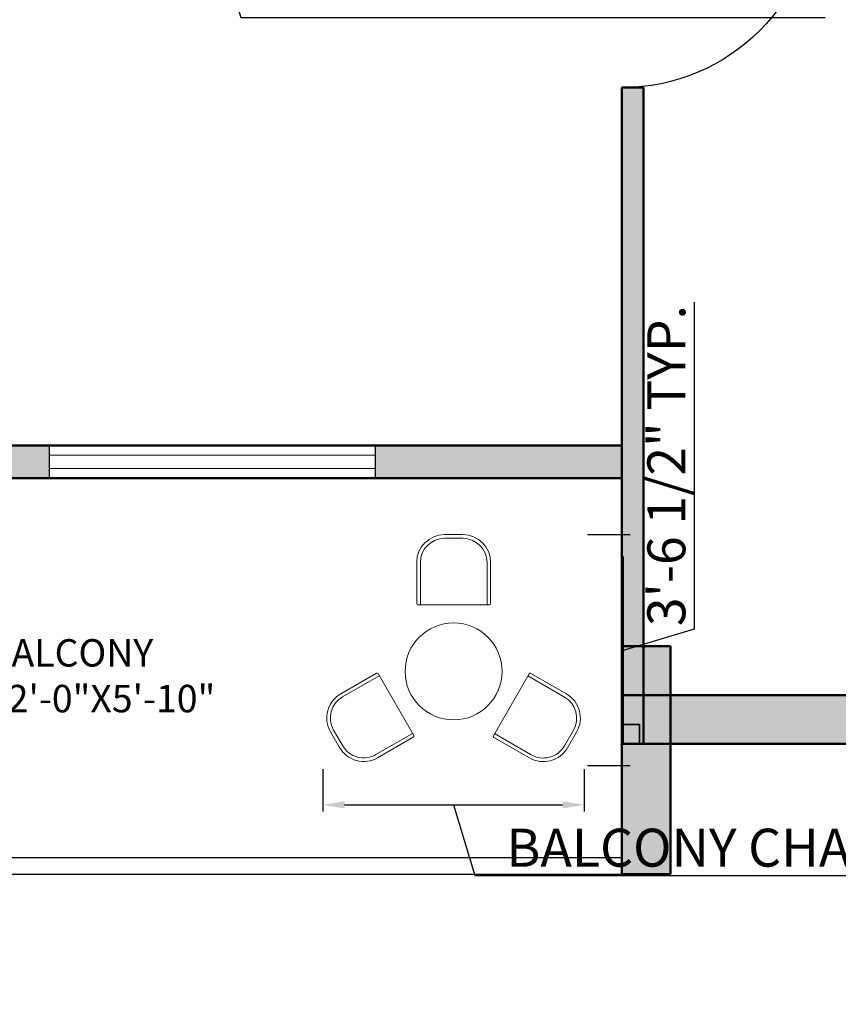
# Model space of a CAD drawing. Units: inches. Extents: x -7 to 1228, y -146 to 1091.
# Tile 15 of 88: x 269 to 420, y 12 to 194. Entities that reach past the tile are written whole.
import ezdxf

# ---------------------------------------------------------------- set-up
doc = ezdxf.new("R2010")
doc.units = ezdxf.units.IN
for name, color, linetype, lineweight in [('A-ANNO-DIMS', 2, 'Continuous', 18), ('A-AREA-IDEN', 7, 'Continuous', 18), ('A-COLS', 6, 'Continuous', 35), ('A-DOOR', 4, 'Continuous', 25), ('A-FURN', 8, 'Continuous', 18), ('A-GLAZ', 175, 'Continuous', 25), ('A-WALL', 7, 'Continuous', 50), ('A-WALL-PATT', 251, 'Continuous', 13)]:
    doc.layers.add(name, color=color, linetype=linetype, lineweight=lineweight)
doc.styles.get("Standard").update_dxf_attribs({"font": 'arial.ttf'})
doc.dimstyles.new('ISO-25', dxfattribs={"dimtxt": 7, "dimasz": 4, "dimexe": 1.25, "dimexo": 0.625, "dimtad": 1, "dimdec": 1, "dimlunit": 3, "dimtxsty": 'Standard', "dimcen": 2.5, "dimadec": 0, "dimazin": 0, "dimtfac": 1, "dimtdec": 1, "dimtmove": 1, "dimatfit": 3, "dimfxl": 1, "dimarcsym": 0})

# ---------------------------------------------------------------- blocks, each defined once
blk = doc.blocks.new('A$C670C3AF2')
for p, q in [((1122.2, 1874.5), (972.2, 1874.5)), ((1122.2, 1844.5), (972.2, 1844.5)), ((742.2, 1644.5), (742.2, 1304.5)), ((772.2, 1644.5), (772.2, 1294.5)), ((1322.2, 1294.5), (1322.2, 1644.5)), ((1352.2, 1304.5), (1352.2, 1644.5)), ((752.2, 1294.5), (1342.2, 1294.5)), ((409, 730), (114.5, 560)), ((432.6, 709), (129.5, 534)), ((717.6, 215.4), (422.6, 726.3)), ((1669.5, 724.9), (1374.5, 214)), ((1962.6, 532.6), (1659.5, 707.6)), ((1977.6, 558.6), (1683.1, 728.6)), ((30.3, 245.8), (105.3, 115.9)), ((56.3, 260.8), (131.3, 130.9)), ((1960.8, 129.5), (2035.8, 259.4)), ((1986.8, 114.5), (2061.8, 244.4)), ((404.5, 57.7), (707.6, 232.7)), ((419.5, 31.7), (714, 201.7)), ((1378.1, 200.3), (1672.6, 30.3)), ((1384.5, 231.3), (1687.6, 56.3))]:
    blk.add_line(p, q)
blk.add_circle((1046.4, 744.9), 400)
for centre, radius, start, end in [((972.2, 1644.5), 230, 90, 180), ((1122.2, 1644.5), 230, 0, 90), ((972.2, 1644.5), 200, 90, 180), ((1122.2, 1644.5), 200, 0, 90), ((752.2, 1304.5), 10, 180, 270), ((1342.2, 1304.5), 10, 270, 0), ((414, 721.3), 10, 30, 120), ((1678.1, 719.9), 10, 60, 150), ((229.5, 360.8), 230, 120, 210), ((229.5, 360.8), 200, 120, 210), ((1862.6, 359.4), 200, 330, 60), ((1862.6, 359.4), 230, 330, 60), ((709, 210.4), 10, 300, 30), ((1383.1, 209), 10, 150, 240), ((304.5, 230.9), 230, 210, 300), ((304.5, 230.9), 200, 210, 300), ((1787.6, 229.5), 230, 240, 330), ((1787.6, 229.5), 200, 240, 330)]:
    blk.add_arc(centre, radius, start, end)
blk = doc.blocks.new('WIN-BALCONY-60')
for p, q in [((0, 0), (0, 6)), ((0, 6), (60, 6)), ((60, 6), (60, 0)), ((0, 4.29), (60, 4.29)), ((60, 4.29), (60, 1.76)), ((60, 1.76), (0, 1.76)), ((60, 0), (0, 0))]:
    blk.add_line(p, q)
blk = doc.blocks.new('DOOR-900')
blk.add_line((36, 0), (36, 36))
blk.add_arc((36, 0), 36, 90, 180)
blk = doc.blocks.new('*D36')
at = {"layer": 'A-ANNO-DIMS', "color": 0, "lineweight": -2, "transparency": 16777216}
for p, q in [((270.86, 216.83), (270.86, 205.7)), ((340.87, 216.83), (340.87, 205.7)), ((274.86, 206.95), (336.87, 206.95)), ((305.87, 206.95), (309.78, 193.91)), ((309.78, 193.91), (417.47, 193.91))]:
    blk.add_line(p, q, dxfattribs=at)
at = {"layer": 'A-ANNO-DIMS', "color": 0, "transparency": 16777216}
for points in [[(274.86, 207.62), (274.86, 206.28), (270.86, 206.95)], [(336.87, 207.62), (336.87, 206.28), (340.87, 206.95)]]:
    blk.add_solid(points, dxfattribs=at)
at = {"layer": 'Defpoints', "color": 0, "transparency": 16777216}
for p in [(270.86, 217.45), (340.87, 217.45), (340.87, 206.95)]:
    blk.add_point(p, dxfattribs=at)
at = {"layer": 'A-ANNO-DIMS', "color": 0, "transparency": 16777216, "insert": (363.62, 198.15), "char_height": 7, "attachment_point": 5}
blk.add_mtext('DINING SET 5\'-10" TYP.', dxfattribs=at)
blk = doc.blocks.new('*D38')
at = {"layer": 'A-ANNO-DIMS', "color": 0, "lineweight": -2, "transparency": 16777216}
for p, q in [((324.91, 55.36), (324.91, 47.51)), ((373.1, 55.36), (373.1, 47.51)), ((328.91, 48.76), (369.1, 48.76)), ((349, 48.76), (352.92, 35.7)), ((352.92, 35.7), (500.86, 35.7))]:
    blk.add_line(p, q, dxfattribs=at)
at = {"layer": 'A-ANNO-DIMS', "color": 0, "transparency": 16777216}
for points in [[(328.91, 49.42), (328.91, 48.09), (324.91, 48.76)], [(369.1, 49.42), (369.1, 48.09), (373.1, 48.76)]]:
    blk.add_solid(points, dxfattribs=at)
at = {"layer": 'Defpoints', "color": 0, "transparency": 16777216}
for p in [(324.91, 55.99), (373.1, 55.99), (373.1, 48.76)]:
    blk.add_point(p, dxfattribs=at)
at = {"layer": 'A-ANNO-DIMS', "color": 0, "transparency": 16777216, "insert": (426.89, 39.95), "char_height": 7, "attachment_point": 5}
blk.add_mtext('BALCONY CHAIR SET 4\'-0" TYP.', dxfattribs=at)
blk = doc.blocks.new('*D39')
at = {"layer": 'A-ANNO-DIMS', "color": 0, "lineweight": -2, "transparency": 16777216}
for p, q in [((393.38, 81.2), (393.38, 141.42)), ((373.72, 98.58), (381.58, 98.58)), ((380.33, 59.99), (380.33, 94.58)), ((380.33, 77.28), (393.38, 81.2)), ((373.72, 55.99), (381.58, 55.99))]:
    blk.add_line(p, q, dxfattribs=at)
at = {"layer": 'A-ANNO-DIMS', "color": 0, "transparency": 16777216}
for points in [[(379.66, 94.58), (380.99, 94.58), (380.33, 98.58)], [(379.66, 59.99), (380.99, 59.99), (380.33, 55.99)]]:
    blk.add_solid(points, dxfattribs=at)
at = {"layer": 'Defpoints', "color": 0, "transparency": 16777216}
for p in [(373.1, 98.58), (380.33, 98.58), (373.1, 55.99)]:
    blk.add_point(p, dxfattribs=at)
at = {"layer": 'A-ANNO-DIMS', "color": 0, "transparency": 16777216, "insert": (389.13, 111.31), "char_height": 7, "attachment_point": 5, "rotation": 90}
blk.add_mtext('3\'-6 1/2" TYP.', dxfattribs=at)

msp = doc.modelspace()

# ---------------------------------------------------------------- hatches: boundary and pattern name
at = {"layer": 'A-COLS'}
h = msp.add_hatch(color=256, dxfattribs=at)
h.dxf.hatch_style = 1
h.paths.add_polyline_path([(380, 63.55), (383.29, 63.55), (383.29, 60), (389, 60), (389, 78), (380, 78)])
h = msp.add_hatch(color=256, dxfattribs=at)
h.dxf.hatch_style = 1
h.paths.add_polyline_path([(380, 63.55), (380, 60), (383.29, 60), (383.29, 63.55)])
at = {"layer": 'A-WALL-PATT'}
h = msp.add_hatch(color=256, dxfattribs=at)
h.dxf.hatch_style = 1
h.paths.add_polyline_path([(69, 568), (60, 568), (60, 493), (63.29, 493), (69, 493)])
h.paths.add_polyline_path([(69, 662.41), (60, 662.41), (60, 586), (69, 586)], flags=17)
h.paths.add_polyline_path([(69, 723), (184, 723), (184, 734), (179, 734), (179, 728), (69, 728), (69, 741.62), (60, 741.62), (60, 698.41), (69, 698.41)], flags=17)
h.paths.add_polyline_path([(69, 782), (231, 782), (231, 728), (231, 723), (231, 586), (236, 586), (236, 787), (69, 787), (69, 800.13), (60, 800.13), (60, 765.62), (69, 765.62)])
h.paths.add_polyline_path([(184, 842), (189, 842), (189, 848), (173, 848), (173, 842), (179, 842), (179, 787), (184, 787)])
h.paths.add_polyline_path([(118.22, 69), (69, 69), (69, 60), (118.22, 60)])
h.paths.add_polyline_path([(227, 69), (154.22, 69), (154.22, 60), (227, 60)])
h.paths.add_polyline_path([(236, 60), (232.71, 60), (227, 60), (227, 36), (236, 36)])
h.paths.add_polyline_path([(389, 60), (380, 60), (380, 36), (389, 36)])
h.paths.add_polyline_path([(384, 181), (380, 181), (380, 115), (380, 78), (384, 78)])
h.paths.add_polyline_path([(380, 115), (334.55, 115), (334.55, 109), (380, 109)])
h.paths.add_polyline_path([(274.55, 115), (236, 115), (236, 201), (232.71, 201), (231, 201), (231, 78), (236, 78), (236, 109), (274.55, 109)])
h.paths.add_polyline_path([(69, 123), (60, 123), (60, 78), (69, 78)])
h.paths.add_polyline_path([(69, 201), (60, 201), (60, 159), (69, 159)])
h.paths.add_polyline_path([(143, 219), (69, 219), (69, 213), (143, 213)], flags=17)
h.paths.add_polyline_path([(189, 219), (184, 219), (184, 274), (231, 274), (231, 219), (236, 219), (236, 279), (184, 279), (184, 297), (179, 297), (179, 279), (69, 279), (69, 290.91), (60, 290.91), (60, 262.18), (69, 262.18), (69, 274), (179, 274), (179, 219), (173, 219), (173, 213), (189, 213)])
h.paths.add_polyline_path([(69, 238.18), (60, 238.18), (60, 219), (69, 219)], flags=17)
h.paths.add_polyline_path([(69, 333), (60, 333), (60, 314.91), (69, 314.91), (69, 316.96)])
h.paths.add_polyline_path([(190, 338), (184, 338), (69, 338), (69, 333), (179, 333), (179, 327), (184, 327), (184, 333.02), (190, 333.05)])
h.paths.add_polyline_path([(69, 386.81), (60, 386.81), (60, 351), (69, 351)])
h.paths.add_polyline_path([(69, 475), (60, 475), (60, 422.81), (69, 422.81)])
h.paths.add_polyline_path([(236, 475), (231, 475), (231, 351.24), (236, 351.24)])
h.paths.add_polyline_path([(384, 475), (380, 475), (380, 362), (384, 362)])
h.paths.add_polyline_path([(547, 307), (439, 307), (439, 356), (445, 356), (445, 362), (433, 362), (433, 307), (380, 307), (380, 244), (380, 241), (384, 241), (384, 301), (433, 301), (433, 277), (439, 277), (439, 301), (547, 301)])
h.paths.add_polyline_path([(547, 241), (439, 241), (439, 247), (433, 247), (433, 235), (547, 235)])
h.paths.add_polyline_path([(450, 69), (440.29, 69), (424.89, 69), (389, 69), (389, 60), (450, 60)])
h.paths.add_polyline_path([(547, 69), (486, 69), (486, 60), (547, 60)])
h.paths.add_polyline_path([(556, 148.27), (547, 148.27), (547, 78), (556, 78)])
h.paths.add_polyline_path([(556, 223), (547, 223), (547, 195), (547, 184.27), (556, 184.27)])
h.paths.add_polyline_path([(556, 311.19), (547, 311.19), (547, 273.08), (556, 273.08)])
h.paths.add_polyline_path([(556, 344), (552.71, 344), (547, 344), (547, 335.19), (556, 335.19)])
h.paths.add_polyline_path([(556, 249.08), (547, 249.08), (547, 241), (556, 241)])
h.paths.add_polyline_path([(547, 362), (475, 362), (475, 356), (547, 356)], flags=0)
h.paths.add_polyline_path([(556, 399.62), (547, 399.62), (547, 362), (556, 362)])
h.paths.add_polyline_path([(556, 475), (547, 475), (547, 435.62), (556, 435.62)])
h.paths.add_polyline_path([(547, 493), (389, 493), (389, 487), (547, 487)])
h.paths.add_polyline_path([(380, 493), (278, 493), (278, 487), (380, 487)])
h.paths.add_polyline_path([(227, 493), (69, 493), (69, 487), (227, 487)])
h.paths.add_polyline_path([(643, 122.44), (634, 122.44), (634, 78), (643, 78)])
h.paths.add_polyline_path([(702.5, 69), (692.79, 69), (677.39, 69), (643, 69), (643, 60), (702.5, 60)])
h.paths.add_polyline_path([(798, 69), (738.5, 69), (738.5, 60), (798, 60)])
h.paths.add_polyline_path([(807, 60), (803.71, 60), (798, 60), (798, 36), (807, 36)])
h.paths.add_polyline_path([(807, 109), (846.75, 109), (846.75, 115), (807, 115), (807, 159), (802, 159), (802, 78), (807, 78)])
h.paths.add_polyline_path([(807, 201), (802, 201), (802, 195), (807, 195)])
h.paths.add_polyline_path([(643, 201), (634, 201), (634, 158.44), (643, 158.44)])
h.paths.add_polyline_path([(756, 225), (751, 225), (751, 219), (643, 219), (643, 213), (756, 213)])
h.paths.add_polyline_path([(643, 240.85), (634, 240.85), (634, 219), (643, 219)])
h.paths.add_polyline_path([(643, 274), (643, 288.63), (634, 288.63), (634, 264.85), (643, 264.85)])
h.paths.add_polyline_path([(802, 279), (756, 279), (756, 297), (751, 297), (751, 279), (643, 279), (643, 274), (751, 274), (751, 255), (756, 255), (756, 274), (802, 274)])
h.paths.add_polyline_path([(807, 333), (803.71, 333), (802, 333), (802, 279), (802, 274), (802, 219), (807, 219)])
h.paths.add_polyline_path([(956, 182), (951, 182), (951, 115), (906.75, 115), (906.75, 109), (951, 109), (951, 78), (956, 78)])
h.paths.add_polyline_path([(960, 60), (951, 60), (951, 36), (960, 36)])
h.paths.add_polyline_path([(1021, 69), (1005.78, 69), (960, 69), (960, 60), (1021, 60)])
h.paths.add_polyline_path([(956, 224), (951, 224), (951, 218), (956, 218)])
h.paths.add_polyline_path([(956, 302), (1004, 302), (1004, 278), (1010, 278), (1010, 302), (1118, 302), (1118, 290.81), (1127, 290.81), (1127, 326.97), (1118, 326.97), (1118, 320.97), (1118, 307), (1010, 307), (1010, 356), (1016, 356), (1016, 362), (1004, 362), (1004, 307), (951, 307), (951, 244), (951, 242), (954.29, 242), (956, 242)])
h.paths.add_polyline_path([(643, 333), (634, 333), (634, 312.63), (643, 312.63), (643, 316.96)])
h.paths.add_polyline_path([(756, 338), (643, 338), (643, 333), (751, 333), (751, 327), (756, 327)])
h.paths.add_polyline_path([(643, 388), (634, 388), (634, 351), (643, 351)])
h.paths.add_polyline_path([(807, 357), (802, 357), (802, 351), (807, 351)])
h.paths.add_polyline_path([(807, 475), (802, 475), (802, 393), (807, 393)])
h.paths.add_polyline_path([(643, 475), (634, 475), (634, 424), (643, 424)])
h.paths.add_polyline_path([(798, 493), (643, 493), (643, 487), (798, 487)])
h.paths.add_polyline_path([(634, 493), (556, 493), (556, 487), (634, 487)])
h.paths.add_polyline_path([(813, 493), (807, 493), (807, 487), (813, 487)])
h.paths.add_polyline_path([(951, 493), (849, 493), (849, 487), (951, 487)])
h.paths.add_polyline_path([(956, 484), (951, 484), (951, 374), (956, 374)])
h.paths.add_polyline_path([(1109, 493), (969, 493), (969, 487), (1109, 487)])
h.paths.add_polyline_path([(1127, 484), (1118, 484), (1118, 450.64), (1127, 450.64)])
h.paths.add_polyline_path([(1127, 414.64), (1118, 414.64), (1118, 365), (1127, 365)])
h.paths.add_polyline_path([(1109, 362), (1046, 362), (1046, 356), (1109, 356)], flags=17)
h.paths.add_polyline_path([(1127, 356), (1123.45, 356), (1118, 356), (1118, 350.97), (1127, 350.97)], flags=0)
h.paths.add_polyline_path([(1127, 266.81), (1118, 266.81), (1118, 262.36), (1118, 242), (1127, 242)], flags=17)
h.paths.add_polyline_path([(1118, 242), (1010, 242), (1010, 248), (1004, 248), (1004, 237), (1118, 237)])
h.paths.add_polyline_path([(1127, 224), (1118, 224), (1118, 170), (1127, 170)])
h.paths.add_polyline_path([(1127, 134), (1118, 134), (1118, 78), (1127, 78)])
h.paths.add_polyline_path([(1118, 69), (1057, 69), (1057, 60), (1118, 60)])
h.paths.add_polyline_path([(227, 571.55), (227, 574), (69, 574), (69, 568), (227, 568)])
h.paths.add_polyline_path([(380, 571.55), (380, 574), (278, 574), (278, 568), (380, 568)])
h.paths.add_polyline_path([(242, 574), (236, 574), (236, 568), (242, 568)])
h.paths.add_polyline_path([(547, 571.55), (547, 574), (389, 574), (389, 568), (547, 568)])
h.paths.add_polyline_path([(384, 733), (380, 733), (380, 586), (384, 586)])
h.paths.add_polyline_path([(556, 646), (634, 646), (634, 655), (547, 655), (547, 586), (556, 586)])
h.paths.add_polyline_path([(634, 574), (556, 574), (556, 568), (634, 568)])
h.paths.add_polyline_path([(643, 655), (634, 655), (634, 586), (643, 586)])
h.paths.add_polyline_path([(798, 574), (643, 574), (643, 568), (798, 568)])
h.paths.add_polyline_path([(643, 663.85), (634, 663.85), (634, 655), (643, 655)])
h.paths.add_polyline_path([(556, 676.97), (547, 676.97), (547, 655), (556, 655)])
h.paths.add_polyline_path([(556, 733), (547, 733), (547, 712.97), (556, 712.97)])
h.paths.add_polyline_path([(643, 710), (634, 710), (634, 699.85), (643, 699.85)])
h.paths.add_polyline_path([(807, 668), (802, 668), (802, 586), (807, 586)])
h.paths.add_polyline_path([(951, 574), (849, 574), (849, 568), (951, 568)])
h.paths.add_polyline_path([(956, 691), (951, 691), (951, 577), (956, 577)])
h.paths.add_polyline_path([(1109, 574), (969, 574), (969, 568), (1109, 568)])
h.paths.add_polyline_path([(1127, 643.4), (1118, 643.4), (1118, 577), (1127, 577)])
h.paths.add_polyline_path([(1127, 568), (1123.45, 568), (1118, 568), (1118, 493), (1127, 493)])
h.paths.add_polyline_path([(1127, 733), (1118, 733), (1118, 679.4), (1127, 679.4)])
h.paths.add_polyline_path([(1127, 777.35), (1118, 777.35), (1118, 770.04), (1118, 751), (1127, 751)], flags=17)
h.paths.add_polyline_path([(1118, 751), (1010, 751), (1010, 757), (1004, 757), (1004, 745), (1118, 745)])
h.paths.add_polyline_path([(956, 811), (1004, 811), (1004, 787), (1010, 787), (1010, 811), (1017.87, 811), (1017.87, 811.63, -0.414214), (1018.25, 812), (1031.98, 812, -0.414214), (1032.35, 811.63), (1032.35, 811), (1118, 811), (1118, 801.35), (1127, 801.35), (1127, 834.69), (1118, 834.69), (1118, 830.24), (1118, 817), (1010, 817), (1010, 866), (1016, 866), (1016, 872), (1004, 872), (1004, 817), (956, 817), (956, 866), (951, 866), (951, 751), (954.29, 751), (956, 751)])
h.paths.add_polyline_path([(1118, 872), (1046, 872), (1046, 866), (1118, 866)], flags=17)
h.paths.add_polyline_path([(1127, 924.71), (1118, 924.71), (1118, 884), (1127, 884)])
h.paths.add_polyline_path([(1127, 866), (1123.71, 866), (1118, 866), (1118, 858.69), (1127, 858.69)], flags=17)
h.paths.add_polyline_path([(956, 983), (951, 983), (951, 952), (807, 952), (807, 983), (802, 983), (802, 902), (807, 902), (807, 946), (951, 946), (951, 884), (956, 884)])
h.paths.add_polyline_path([(807, 842), (802, 842), (802, 787), (756, 787), (756, 806), (751, 806), (751, 787), (643, 787), (643, 782), (751, 782), (751, 764), (756, 764), (756, 782), (802, 782), (802, 728), (807, 728)])
h.paths.add_polyline_path([(756, 848), (643, 848), (643, 842), (751, 842), (751, 836), (756, 836)])
h.paths.add_polyline_path([(756, 734), (751, 734), (751, 728), (643, 728), (643, 723), (756, 723)])
h.paths.add_polyline_path([(643, 749.79), (634, 749.79), (634, 728), (637.29, 728), (643, 728)])
h.paths.add_polyline_path([(643, 805.41), (634, 805.41), (634, 773.79), (643, 773.79)])
h.paths.add_polyline_path([(643, 896.66), (634, 896.66), (634, 860), (637.29, 860), (643, 860)])
h.paths.add_polyline_path([(643, 842), (634, 842), (634, 829.41), (643, 829.41)])
h.paths.add_polyline_path([(643, 983), (634, 983), (634, 932.66), (643, 932.66)])
h.paths.add_polyline_path([(1127, 983), (1118, 983), (1118, 960.71), (1127, 960.71)])
h.paths.add_polyline_path([(1118, 1001), (1077.53, 1001), (1077.53, 992), (1118, 992)])
h.paths.add_polyline_path([(1041.53, 1001), (960, 1001), (960, 992), (1041.53, 992)])
h.paths.add_polyline_path([(960, 1025), (951, 1025), (951, 1001), (954.29, 1001), (960, 1001)])
h.paths.add_polyline_path([(807, 1025), (798, 1025), (798, 1001), (807, 1001)])
h.paths.add_polyline_path([(798, 1001), (738.5, 1001), (738.5, 992), (798, 992)])
h.paths.add_polyline_path([(702.5, 1001), (643, 1001), (643, 992), (702.5, 992)])
h.paths.add_polyline_path([(547, 1001), (499.11, 1001), (499.11, 992), (547, 992)])
h.paths.add_polyline_path([(463.11, 1001), (389, 1001), (389, 992), (463.11, 992)])
h.paths.add_polyline_path([(389, 1025), (380, 1025), (380, 1022), (380, 1001), (383.29, 1001), (389, 1001)])
h.paths.add_polyline_path([(236, 1025), (227, 1025), (227, 1001), (236, 1001)])
h.paths.add_polyline_path([(236, 983), (231, 983), (231, 860), (236, 860)])
h.paths.add_polyline_path([(274.55, 952), (236, 952), (236, 946), (274.55, 946)])
h.paths.add_polyline_path([(380, 952), (334.55, 952), (334.55, 946), (380, 946)])
h.paths.add_polyline_path([(384, 983), (380, 983), (380, 884), (383.29, 884), (384, 884)])
h.paths.add_polyline_path([(227, 1001), (155.01, 1001), (155.01, 992), (162.87, 992), (227, 992)])
h.paths.add_polyline_path([(119.01, 1001), (69, 1001), (69, 992), (119.01, 992)])
h.paths.add_polyline_path([(69, 983), (60, 983), (60, 922.99), (69, 922.99)])
h.paths.add_polyline_path([(69, 886.99), (60, 886.99), (60, 860), (63.29, 860), (69, 860)])
h.paths.add_polyline_path([(143, 848), (69, 848), (69, 842), (143, 842)])

# ---------------------------------------------------------------- linework, layer by layer
at = {"layer": 'A-COLS'}
msp.add_lwpolyline([(380, 60), (383.29, 60), (383.29, 63.55), (380, 63.55)], close=True, dxfattribs=at)
at = {"layer": 'A-GLAZ'}
for p, q in [((380, 39), (236, 39)), ((236, 36), (380, 36))]:
    msp.add_line(p, q, dxfattribs=at)
at = {"layer": 'A-WALL'}
for p, q in [((384, 181), (380, 181)), ((380, 181), (380, 60)), ((380, 115), (380, 181)), ((384, 60), (384, 181)), ((384, 181), (384, 60)), ((380, 115), (236, 115)), ((380, 109), (236, 109)), ((380, 60), (380, 109)), ((389, 78), (380, 78)), ((380, 78), (380, 60)), ((389, 60), (389, 78)), ((556, 69), (380, 69)), ((556, 60), (380, 60)), ((380, 60), (380, 36)), ((380, 60), (389, 60)), ((380, 60), (807, 60)), ((389, 36), (389, 60)), ((380, 36), (380, 39)), ((380, 36), (389, 36))]:
    msp.add_line(p, q, dxfattribs=at)

# ---------------------------------------------------------------- block references
at = {"layer": 'A-DOOR', "extrusion": (0, 0, -1), "zscale": -1, "rotation": 89.99999999999969}
msp.add_blockref('DOOR-900', (-380, 181), dxfattribs=at)
at = {"layer": 'A-FURN', "xscale": 0.022327308386288, "yscale": 0.022327308386288, "zscale": 0.022327308386288}
msp.add_blockref('A$C670C3AF2', (325.65, 56.73), dxfattribs=at)
at = {"layer": 'A-GLAZ', "rotation": 359.964472723119}
msp.add_blockref('WIN-BALCONY-60', (274.55, 109), dxfattribs=at)

# ---------------------------------------------------------------- texts
at = {"layer": 'A-AREA-IDEN', "insert": (263.01, 79.31), "char_height": 5.0568, "attachment_point": 1}
msp.add_mtext_dynamic_manual_height_columns('BALCONY\\P12\'-0"X5\'-10"', width=137.2821, gutter_width=25.28, heights=[0], dxfattribs=at)

# ---------------------------------------------------------------- dimensions: what is measured, and where the dimension line sits
at = {"layer": 'A-ANNO-DIMS'}
for base, p1, p2, text, picture, middle in [((340.87, 206.95), (270.86, 217.45), (340.87, 217.45), 'DINING SET <> TYP.', '*D36', (310.4, 198.15)), ((373.1, 48.76), (324.91, 55.99), (373.1, 55.99), 'BALCONY CHAIR SET <> TYP.', '*D38', (353.54, 39.95))]:
    dim = msp.add_linear_dim(base=base, p1=p1, p2=p2, text=text, dimstyle='ISO-25', override={"dimdec": 1, "dimlfac": 1, "dimrnd": 0, "dimzin": 1, "dimdsep": 46, "dimlunit": 4, "dimfrac": 2}, dxfattribs=at)
    dim.commit()
    dim.dimension.update_dxf_attribs({"geometry": picture, "text_midpoint": middle})
dim = msp.add_linear_dim(base=(380.33, 98.58), p1=(373.1, 55.99), p2=(373.1, 98.58), angle=90, text='<> TYP.', dimstyle='ISO-25', override={"dimdec": 1, "dimlfac": 1, "dimrnd": 0, "dimzin": 1, "dimdsep": 46, "dimlunit": 4, "dimfrac": 2}, dxfattribs=at)
dim.commit()
dim.dimension.update_dxf_attribs({"geometry": '*D39', "text_midpoint": (389.13, 81.82)})

doc.saveas('drawing.dxf')
